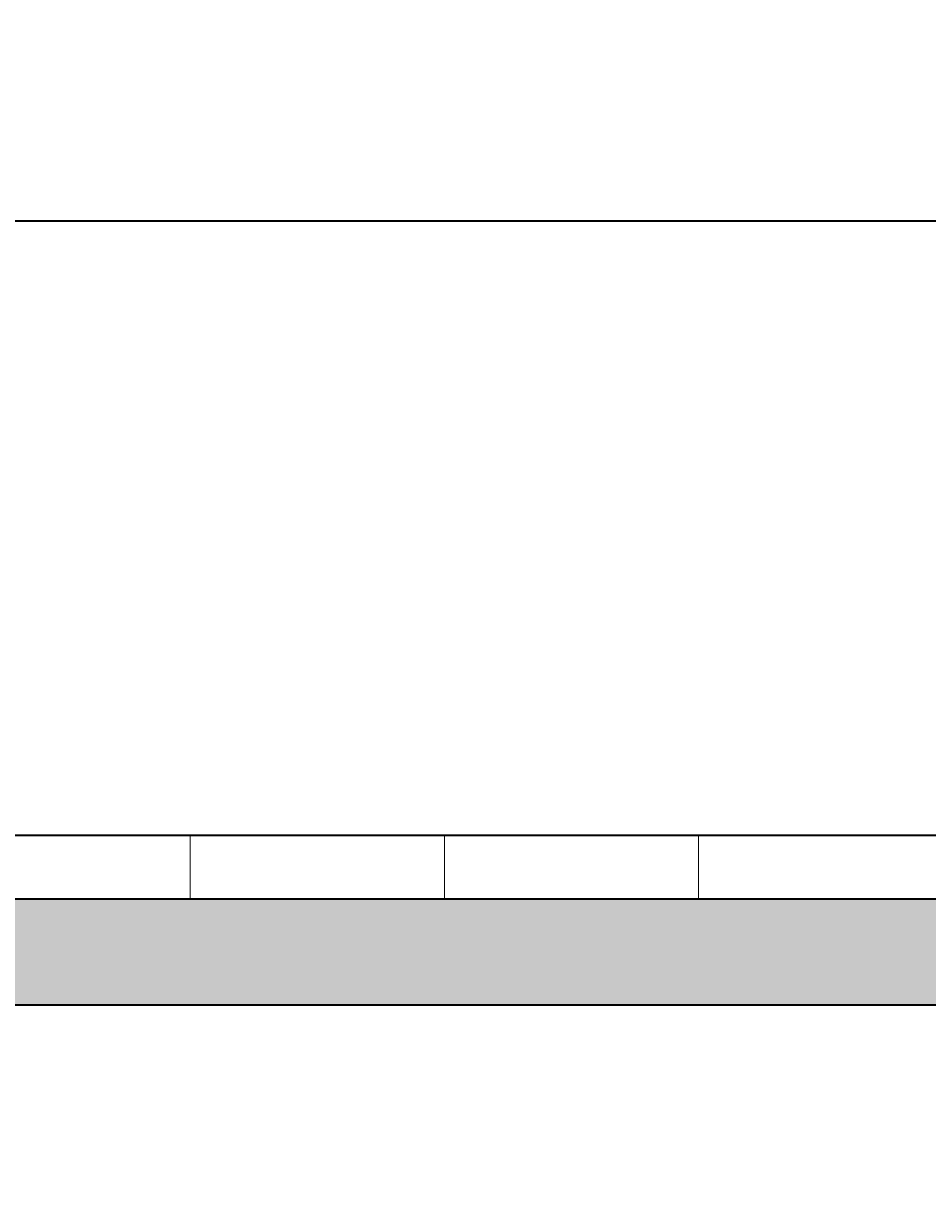
# Model space of a CAD drawing. Units: inches. Extents: x -301 to 715, y -607 to 364.
# Tile 46 of 141: x 64 to 107, y -370 to -315. Entities that reach past the tile are written whole.
import ezdxf

# ---------------------------------------------------------------- set-up
doc = ezdxf.new("R2010")
doc.units = ezdxf.units.IN
doc.header["$MEASUREMENT"] = 0
for name, color, linetype, lineweight in [('A-ANNO-DIMS', 2, 'Continuous', 18), ('A-SECT', 1, 'Continuous', 35), ('A-SECT-PATT', 8, 'Continuous', 13)]:
    doc.layers.add(name, color=color, linetype=linetype, lineweight=lineweight)
doc.styles.get("Standard").update_dxf_attribs({"font": 'arial.ttf'})
doc.dimstyles.get("Standard").update_dxf_attribs({"dimtxt": 0.18, "dimasz": 0.18, "dimexe": 0.18, "dimexo": 0.0625, "dimgap": 0.09, "dimtad": 0, "dimtih": 1, "dimtoh": 1, "dimdec": 1, "dimzin": 0, "dimdsep": 46, "dimlunit": 4, "dimtxsty": 'Standard', "dimcen": 0.09, "dimclrd": 3, "dimclre": 4, "dimclrt": 6, "dimadec": 0, "dimazin": 0, "dimtfac": 1, "dimtdec": 1, "dimtofl": 0, "dimtmove": 0, "dimatfit": 3, "dimfxl": 1, "dimtfill": 2, "dimtfillclr": 51, "dimtolj": 1, "dimtzin": 0, "dimarcsym": 0})

# ---------------------------------------------------------------- blocks, each defined once
blk = doc.blocks.new('*D175')
at = {"layer": 'A-ANNO-DIMS', "color": 4, "lineweight": -2, "transparency": 16777216}
for p, q in [((-199.282, -324.415), (-199.282, -292.467)), ((148.218, -324.415), (148.218, -292.467))]:
    blk.add_line(p, q, dxfattribs=at)
at = {"layer": 'A-ANNO-DIMS', "color": 3, "lineweight": -2, "transparency": 16777216}
for p, q in [((-199.102, -292.647), (-26.212, -292.647)), ((148.038, -292.647), (-24.852, -292.647))]:
    blk.add_line(p, q, dxfattribs=at)
at = {"layer": 'A-ANNO-DIMS', "color": 3, "transparency": 16777216}
for points in [[(-199.102, -292.617), (-199.102, -292.677), (-199.282, -292.647)], [(148.038, -292.617), (148.038, -292.677), (148.218, -292.647)]]:
    blk.add_solid(points, dxfattribs=at)
at = {"layer": 'Defpoints', "color": 0, "transparency": 16777216}
for p in [(148.218, -292.647), (-199.282, -324.477), (148.218, -324.477)]:
    blk.add_point(p, dxfattribs=at)
at = {"layer": 'A-ANNO-DIMS', "color": 6, "transparency": 16777216, "insert": (-25.532, -292.647), "char_height": 0.18, "attachment_point": 5, "bg_fill": 1, "box_fill_scale": 1.25, "bg_fill_color": 51, "bg_fill_transparency": 0}
blk.add_mtext('\\A1;28\'-11 1/2"', dxfattribs=at)
blk = doc.blocks.new('*D176')
at = {"layer": 'A-ANNO-DIMS', "color": 4, "lineweight": -2, "transparency": 16777216}
for p, q in [((148.28, -324.477), (215.605, -324.477)), ((-15.22, -540.477), (215.605, -540.477))]:
    blk.add_line(p, q, dxfattribs=at)
at = {"layer": 'A-ANNO-DIMS', "color": 3, "lineweight": -2, "transparency": 16777216}
for p, q in [((215.425, -324.657), (215.425, -432.296)), ((215.425, -540.297), (215.425, -432.659))]:
    blk.add_line(p, q, dxfattribs=at)
at = {"layer": 'A-ANNO-DIMS', "color": 3, "transparency": 16777216}
for points in [[(215.395, -324.657), (215.455, -324.657), (215.425, -324.477)], [(215.395, -540.297), (215.455, -540.297), (215.425, -540.477)]]:
    blk.add_solid(points, dxfattribs=at)
at = {"layer": 'Defpoints', "color": 0, "transparency": 16777216}
for p in [(148.218, -324.477), (-15.282, -540.477), (215.425, -540.477)]:
    blk.add_point(p, dxfattribs=at)
at = {"layer": 'A-ANNO-DIMS', "color": 6, "transparency": 16777216, "insert": (215.425, -432.477), "char_height": 0.18, "attachment_point": 5, "bg_fill": 1, "box_fill_scale": 1.25, "bg_fill_color": 51, "bg_fill_transparency": 0}
blk.add_mtext('\\A1;18\'-0"', dxfattribs=at)
blk = doc.blocks.new('*D189')
at = {"layer": 'A-ANNO-DIMS', "color": 4, "lineweight": -2, "transparency": 16777216}
for p, q in [((134.193, -353.477), (-266.112, -353.477)), ((134.193, -361.477), (-266.112, -361.477))]:
    blk.add_line(p, q, dxfattribs=at)
at = {"layer": 'A-ANNO-DIMS', "color": 3, "lineweight": -2, "transparency": 16777216}
for p, q in [((-265.932, -353.657), (-265.932, -357.296)), ((-265.932, -361.297), (-265.932, -357.659))]:
    blk.add_line(p, q, dxfattribs=at)
at = {"layer": 'A-ANNO-DIMS', "color": 3, "transparency": 16777216}
for points in [[(-265.962, -353.657), (-265.902, -353.657), (-265.932, -353.477)], [(-265.962, -361.297), (-265.902, -361.297), (-265.932, -361.477)]]:
    blk.add_solid(points, dxfattribs=at)
at = {"layer": 'Defpoints', "color": 0, "transparency": 16777216}
for p in [(134.255, -353.477), (-265.932, -361.477), (134.255, -361.477)]:
    blk.add_point(p, dxfattribs=at)
at = {"layer": 'A-ANNO-DIMS', "color": 6, "transparency": 16777216, "insert": (-265.932, -357.477), "char_height": 0.18, "attachment_point": 5, "bg_fill": 1, "box_fill_scale": 1.25, "bg_fill_color": 51, "bg_fill_transparency": 0}
blk.add_mtext('\\A1;0\'-8"', dxfattribs=at)

msp = doc.modelspace()

# ---------------------------------------------------------------- hatches: boundary and pattern name
at = {"layer": 'A-SECT-PATT'}
h = msp.add_hatch(dxfattribs=at)
h.set_pattern_fill('ANSI31', color=256, scale=96, angle=45, style=0)
h.paths.add_polyline_path([(-185.282, -356.477), (134.255, -356.477), (134.255, -353.477), (-185.282, -353.477)])
h = msp.add_hatch(dxfattribs=at)
h.set_pattern_fill('AR-CONC', color=256, scale=0.5)
h.set_pattern_definition([(50, (10.3213, 33.8764), (3.586301, -0.31376), [0.375, -4.125]), (355, (10.3213, 33.8764), (-0.693757, 3.76096), [0.3, -3.3]), (100.45144, (10.62, 33.8502), (2.892544, 3.4472), [0.3187, -3.50571]), (46.1842, (10.3213, 34.8764), (5.336207, -0.827596), [0.5625, -6.1875]), (96.6356, (10.766, 34.8074), (4.67331, 4.870593), [0.47805, -5.25857]), (351.1842, (10.321, 34.8764), (4.67331, 4.870593), [0.45, -4.95]), (21, (10.8213, 34.6264), (2.984535, -2.013094), [0.375, -4.125]), (326, (10.8213, 34.6264), (1.216577, 3.62575), [0.3, -3.3]), (71.45144, (11.07, 34.4586), (4.201112, 1.612656), [0.3187, -3.50571]), (37.5, (10.3213, 33.8764), (0.0607993, 1.6644693), [0, -3.26, 0, -3.35, 0, -3.3125]), (7.5, (10.3213, 33.8764), (1.3153477, 1.9720586), [0, -1.91, 0, -3.185, 0, -1.2625]), (327.5, (9.2063, 33.8764), (2.6691122, -0.1127744), [0, -1.25, 0, -3.9, 0, -5.175]), (317.5, (8.7063, 33.8764), (2.915931, 0.500525), [0, -1.625, 0, -2.59, 0, -3.675])])
h.paths.add_polyline_path([(-56.282, -535.477), (-61.282, -535.477), (-61.282, -540.477), (-15.282, -540.477), (-15.282, -535.477), (-20.282, -535.477)])
h.paths.add_polyline_path([(119.255, -535.477), (114.255, -535.477), (114.255, -540.477), (163.255, -540.477), (163.255, -535.477), (158.255, -535.477)])
h.paths.add_polyline_path([(-206.282, -471.477), (-209.282, -471.477), (-209.282, -481.477), (-206.282, -481.477), (-194.282, -481.477), (-194.282, -471.477)])
h.paths.add_polyline_path([(-41.282, -481.477), (-41.282, -471.477), (-185.282, -471.477), (-185.282, -481.477), (-180.282, -481.477)])
h.paths.add_polyline_path([(134.255, -481.477), (134.255, -471.477), (-35.282, -471.477), (-35.282, -481.477), (-30.282, -481.477)])
h.paths.add_polyline_path([(155.218, -481.477), (158.218, -481.477), (158.218, -471.477), (153.218, -471.477), (143.218, -471.477), (143.218, -481.477), (148.255, -481.477)])
h.paths.add_polyline_path([(-193.88, -356.477), (-193.904, -361.477), (143.218, -361.477), (143.218, -356.477)])

# ---------------------------------------------------------------- linework, layer by layer
at = {"layer": 'A-SECT'}
for p, q in [((-185.282, -324.477), (134.255, -324.477)), ((-194.282, -353.477), (143.218, -353.477)), ((-194.282, -356.477), (143.218, -356.477)), ((-194.282, -361.477), (143.218, -361.477))]:
    msp.add_line(p, q, dxfattribs=at)

# ---------------------------------------------------------------- dimensions: what is measured, and where the dimension line sits
at = {"layer": 'A-ANNO-DIMS'}
dim = msp.add_linear_dim(base=(148.218, -292.647), p1=(-199.282, -324.477), p2=(148.218, -324.477), dimstyle='Standard', override={"dimdec": 1, "dimlfac": 1, "dimrnd": 0, "dimzin": 1, "dimdsep": 46, "dimlunit": 4, "dimfrac": 2}, dxfattribs=at)
dim.commit()
dim.dimension.update_dxf_attribs({"geometry": '*D175', "text_midpoint": (-25.532, -292.647)})
for base, p1, p2, picture, middle in [((215.425, -540.477), (148.218, -324.477), (-15.282, -540.477), '*D176', (215.425, -432.477)), ((-265.932, -361.477), (134.255, -353.477), (134.255, -361.477), '*D189', (-265.932, -357.477))]:
    dim = msp.add_linear_dim(base=base, p1=p1, p2=p2, angle=90, dimstyle='Standard', override={"dimdec": 1, "dimlfac": 1, "dimrnd": 0, "dimzin": 1, "dimdsep": 46, "dimlunit": 4, "dimfrac": 2}, dxfattribs=at)
    dim.commit()
    dim.dimension.update_dxf_attribs({"geometry": picture, "text_midpoint": middle})

doc.saveas('drawing.dxf')
